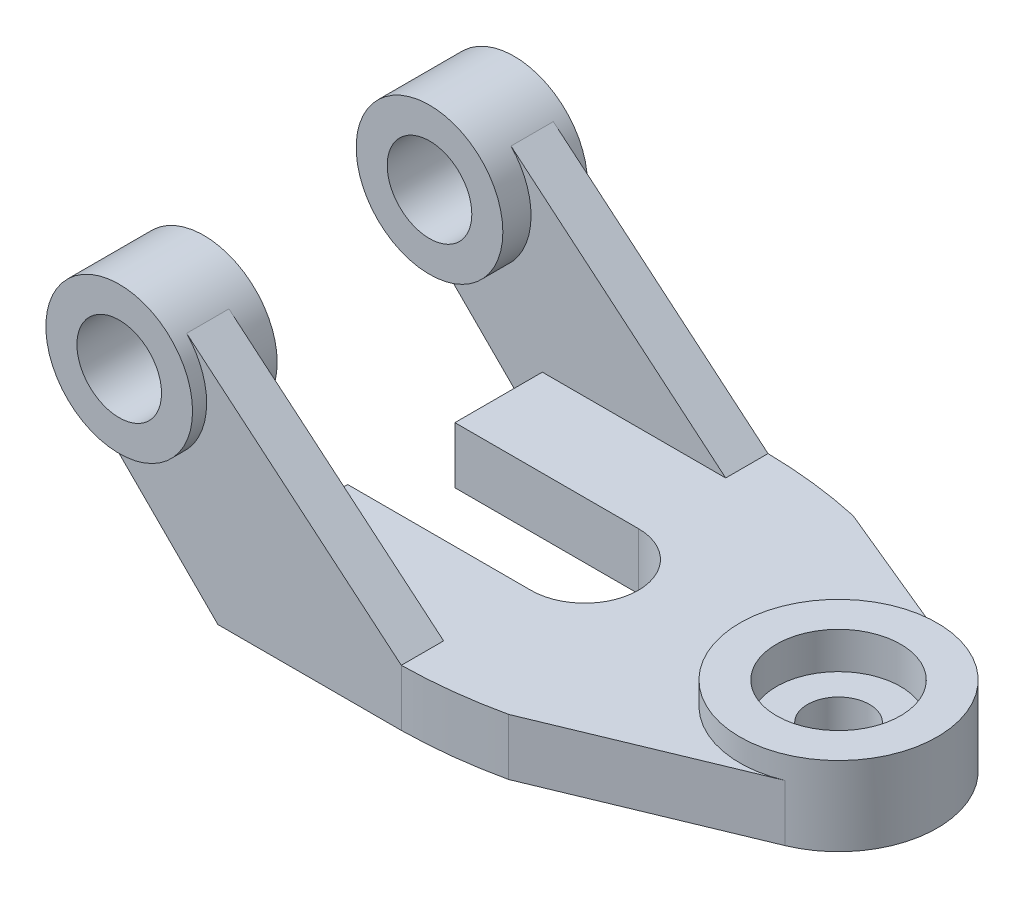
ISO-10303-21;
HEADER;
FILE_DESCRIPTION(('STEP AP214'),'2;1');
FILE_NAME('part.step','',(''),(''),'','','');
FILE_SCHEMA(('AUTOMOTIVE_DESIGN { 1 0 10303 214 1 1 1 1 }'));
ENDSEC;
DATA;
#1=APPLICATION_CONTEXT('core data for automotive mechanical design processes');
#2=APPLICATION_PROTOCOL_DEFINITION('international standard','automotive_design',2000,#1);
#3=PRODUCT_CONTEXT('',#1,'mechanical');
#4=PRODUCT('Part','Part','',(#3));
#5=PRODUCT_RELATED_PRODUCT_CATEGORY('part','',(#4));
#6=PRODUCT_DEFINITION_FORMATION('','',#4);
#7=PRODUCT_DEFINITION_CONTEXT('part definition',#1,'design');
#8=PRODUCT_DEFINITION('design','',#6,#7);
#9=PRODUCT_DEFINITION_SHAPE('','',#8);
#10=(LENGTH_UNIT() NAMED_UNIT(*) SI_UNIT(.MILLI.,.METRE.));
#11=(NAMED_UNIT(*) PLANE_ANGLE_UNIT() SI_UNIT($,.RADIAN.));
#12=(NAMED_UNIT(*) SI_UNIT($,.STERADIAN.) SOLID_ANGLE_UNIT());
#13=UNCERTAINTY_MEASURE_WITH_UNIT(LENGTH_MEASURE(1.E-05),#10,'distance_accuracy_value','');
#14=(GEOMETRIC_REPRESENTATION_CONTEXT(3) GLOBAL_UNCERTAINTY_ASSIGNED_CONTEXT((#13)) GLOBAL_UNIT_ASSIGNED_CONTEXT((#10,
#11,#12)) REPRESENTATION_CONTEXT('',''));
#15=CARTESIAN_POINT('',(0.,0.,0.));
#16=DIRECTION('',(0.,0.,1.));
#17=DIRECTION('',(1.,0.,0.));
#18=AXIS2_PLACEMENT_3D('',#15,#16,#17);
#19=CARTESIAN_POINT('',(-30.,66.,-31.));
#20=DIRECTION('',(0.,0.,-1.));
#21=DIRECTION('',(-1.,0.,0.));
#22=AXIS2_PLACEMENT_3D('',#19,#20,#21);
#23=PLANE('',#22);
#24=CARTESIAN_POINT('',(-30.,66.,-31.));
#25=DIRECTION('',(0.,0.,-1.));
#26=DIRECTION('',(-1.,0.,0.));
#27=AXIS2_PLACEMENT_3D('',#24,#25,#26);
#28=CIRCLE('',#27,26.);
#29=CARTESIAN_POINT('',(-44.2583426132256,44.2583426132257,-31.));
#30=VERTEX_POINT('',#29);
#31=CARTESIAN_POINT('',(-11.1036065621983,83.8585081976016,-31.));
#32=VERTEX_POINT('',#31);
#33=EDGE_CURVE('E379',#30,#32,#28,.F.);
#34=ORIENTED_EDGE('',*,*,#33,.F.);
#35=DIRECTION('',(-0.707106781186546,0.707106781186549,0.));
#36=VECTOR('',#35,1.);
#37=CARTESIAN_POINT('',(0.,0.,-31.));
#38=LINE('',#37,#36);
#39=CARTESIAN_POINT('',(0.,0.,-31.));
#40=VERTEX_POINT('',#39);
#41=EDGE_CURVE('E358',#40,#30,#38,.T.);
#42=ORIENTED_EDGE('',*,*,#41,.F.);
#43=DIRECTION('',(0.,1.,0.));
#44=VECTOR('',#43,1.);
#45=CARTESIAN_POINT('',(0.,20.,-31.));
#46=LINE('',#45,#44);
#47=CARTESIAN_POINT('',(0.,20.,-31.));
#48=VERTEX_POINT('',#47);
#49=EDGE_CURVE('E203',#40,#48,#46,.T.);
#50=ORIENTED_EDGE('',*,*,#49,.T.);
#51=DIRECTION('',(-1.,0.,0.));
#52=VECTOR('',#51,1.);
#53=CARTESIAN_POINT('',(65.,20.,-31.));
#54=LINE('',#53,#52);
#55=CARTESIAN_POINT('',(65.,20.,-31.));
#56=VERTEX_POINT('',#55);
#57=EDGE_CURVE('E56',#56,#48,#54,.T.);
#58=ORIENTED_EDGE('',*,*,#57,.F.);
#59=DIRECTION('',(0.766044443118977,-0.64278760968654,0.));
#60=VECTOR('',#59,1.);
#61=CARTESIAN_POINT('',(65.,20.,-31.));
#62=LINE('',#61,#60);
#63=EDGE_CURVE('E349',#32,#56,#62,.T.);
#64=ORIENTED_EDGE('',*,*,#63,.F.);
#65=EDGE_LOOP('',(#34,#42,#50,#58,#64));
#66=FACE_BOUND('',#65,.T.);
#67=ADVANCED_FACE('F39',(#66),#23,.F.);
#68=CARTESIAN_POINT('',(0.,20.,0.));
#69=DIRECTION('',(1.,0.,0.));
#70=DIRECTION('',(0.,0.,-1.));
#71=AXIS2_PLACEMENT_3D('',#68,#69,#70);
#72=PLANE('',#71);
#73=ORIENTED_EDGE('',*,*,#49,.F.);
#74=DIRECTION('',(0.,0.,1.));
#75=VECTOR('',#74,1.);
#76=CARTESIAN_POINT('',(0.,0.,0.));
#77=LINE('',#76,#75);
#78=CARTESIAN_POINT('',(0.,0.,0.));
#79=VERTEX_POINT('',#78);
#80=EDGE_CURVE('E256',#40,#79,#77,.T.);
#81=ORIENTED_EDGE('',*,*,#80,.T.);
#82=DIRECTION('',(0.,-1.,0.));
#83=VECTOR('',#82,1.);
#84=CARTESIAN_POINT('',(0.,20.,0.));
#85=LINE('',#84,#83);
#86=CARTESIAN_POINT('',(0.,20.,0.));
#87=VERTEX_POINT('',#86);
#88=EDGE_CURVE('E235',#87,#79,#85,.T.);
#89=ORIENTED_EDGE('',*,*,#88,.F.);
#90=DIRECTION('',(0.,0.,1.));
#91=VECTOR('',#90,1.);
#92=CARTESIAN_POINT('',(0.,20.,0.));
#93=LINE('',#92,#91);
#94=EDGE_CURVE('E234',#48,#87,#93,.T.);
#95=ORIENTED_EDGE('',*,*,#94,.F.);
#96=EDGE_LOOP('',(#73,#81,#89,#95));
#97=FACE_BOUND('',#96,.T.);
#98=ADVANCED_FACE('F375',(#97),#72,.F.);
#99=CARTESIAN_POINT('',(0.,20.,38.));
#100=DIRECTION('',(1.,0.,0.));
#101=DIRECTION('',(0.,0.,-1.));
#102=AXIS2_PLACEMENT_3D('',#99,#100,#101);
#103=PLANE('',#102);
#104=DIRECTION('',(0.,-1.,0.));
#105=VECTOR('',#104,1.);
#106=CARTESIAN_POINT('',(0.,20.,69.));
#107=LINE('',#106,#105);
#108=CARTESIAN_POINT('',(0.,20.,69.));
#109=VERTEX_POINT('',#108);
#110=CARTESIAN_POINT('',(0.,0.,69.));
#111=VERTEX_POINT('',#110);
#112=EDGE_CURVE('E189',#109,#111,#107,.T.);
#113=ORIENTED_EDGE('',*,*,#112,.F.);
#114=DIRECTION('',(0.,0.,1.));
#115=VECTOR('',#114,1.);
#116=CARTESIAN_POINT('',(0.,20.,38.));
#117=LINE('',#116,#115);
#118=CARTESIAN_POINT('',(0.,20.,38.));
#119=VERTEX_POINT('',#118);
#120=EDGE_CURVE('E219',#119,#109,#117,.T.);
#121=ORIENTED_EDGE('',*,*,#120,.F.);
#122=DIRECTION('',(0.,-1.,0.));
#123=VECTOR('',#122,1.);
#124=CARTESIAN_POINT('',(0.,20.,38.));
#125=LINE('',#124,#123);
#126=CARTESIAN_POINT('',(0.,0.,38.));
#127=VERTEX_POINT('',#126);
#128=EDGE_CURVE('E283',#119,#127,#125,.T.);
#129=ORIENTED_EDGE('',*,*,#128,.T.);
#130=DIRECTION('',(0.,0.,1.));
#131=VECTOR('',#130,1.);
#132=CARTESIAN_POINT('',(0.,0.,38.));
#133=LINE('',#132,#131);
#134=EDGE_CURVE('E243',#127,#111,#133,.T.);
#135=ORIENTED_EDGE('',*,*,#134,.T.);
#136=EDGE_LOOP('',(#113,#121,#129,#135));
#137=FACE_BOUND('',#136,.T.);
#138=ADVANCED_FACE('F307',(#137),#103,.F.);
#139=CARTESIAN_POINT('',(0.,20.,0.));
#140=DIRECTION('',(0.,0.,-1.));
#141=DIRECTION('',(-1.,0.,0.));
#142=AXIS2_PLACEMENT_3D('',#139,#140,#141);
#143=PLANE('',#142);
#144=DIRECTION('',(1.,0.,0.));
#145=VECTOR('',#144,1.);
#146=CARTESIAN_POINT('',(0.,0.,0.));
#147=LINE('',#146,#145);
#148=CARTESIAN_POINT('',(65.,0.,0.));
#149=VERTEX_POINT('',#148);
#150=EDGE_CURVE('E209',#79,#149,#147,.T.);
#151=ORIENTED_EDGE('',*,*,#150,.T.);
#152=DIRECTION('',(0.,-1.,0.));
#153=VECTOR('',#152,1.);
#154=CARTESIAN_POINT('',(65.,20.,0.));
#155=LINE('',#154,#153);
#156=CARTESIAN_POINT('',(65.,20.,0.));
#157=VERTEX_POINT('',#156);
#158=EDGE_CURVE('E43',#157,#149,#155,.T.);
#159=ORIENTED_EDGE('',*,*,#158,.F.);
#160=DIRECTION('',(1.,0.,0.));
#161=VECTOR('',#160,1.);
#162=CARTESIAN_POINT('',(0.,20.,0.));
#163=LINE('',#162,#161);
#164=EDGE_CURVE('E215',#87,#157,#163,.T.);
#165=ORIENTED_EDGE('',*,*,#164,.F.);
#166=ORIENTED_EDGE('',*,*,#88,.T.);
#167=EDGE_LOOP('',(#151,#159,#165,#166));
#168=FACE_BOUND('',#167,.T.);
#169=ADVANCED_FACE('F41',(#168),#143,.F.);
#170=CARTESIAN_POINT('',(65.,20.,19.));
#171=DIRECTION('',(0.,-1.,0.));
#172=DIRECTION('',(0.,0.,-1.));
#173=AXIS2_PLACEMENT_3D('',#170,#171,#172);
#174=CYLINDRICAL_SURFACE('',#173,19.);
#175=CARTESIAN_POINT('',(65.,0.,19.));
#176=DIRECTION('',(0.,-1.,0.));
#177=DIRECTION('',(0.,0.,1.));
#178=AXIS2_PLACEMENT_3D('',#175,#176,#177);
#179=CIRCLE('',#178,19.);
#180=CARTESIAN_POINT('',(65.,0.,38.));
#181=VERTEX_POINT('',#180);
#182=EDGE_CURVE('E240',#149,#181,#179,.T.);
#183=ORIENTED_EDGE('',*,*,#182,.T.);
#184=DIRECTION('',(0.,-1.,0.));
#185=VECTOR('',#184,1.);
#186=CARTESIAN_POINT('',(65.,20.,38.));
#187=LINE('',#186,#185);
#188=CARTESIAN_POINT('',(65.,20.,38.));
#189=VERTEX_POINT('',#188);
#190=EDGE_CURVE('E281',#189,#181,#187,.T.);
#191=ORIENTED_EDGE('',*,*,#190,.F.);
#192=CARTESIAN_POINT('',(65.,20.,19.));
#193=DIRECTION('',(0.,-1.,0.));
#194=DIRECTION('',(0.,0.,1.));
#195=AXIS2_PLACEMENT_3D('',#192,#193,#194);
#196=CIRCLE('',#195,19.);
#197=EDGE_CURVE('E214',#157,#189,#196,.T.);
#198=ORIENTED_EDGE('',*,*,#197,.F.);
#199=ORIENTED_EDGE('',*,*,#158,.T.);
#200=EDGE_LOOP('',(#183,#191,#198,#199));
#201=FACE_BOUND('',#200,.T.);
#202=ADVANCED_FACE('F295',(#201),#174,.F.);
#203=CARTESIAN_POINT('',(65.,20.,38.));
#204=DIRECTION('',(0.,0.,1.));
#205=DIRECTION('',(1.,0.,0.));
#206=AXIS2_PLACEMENT_3D('',#203,#204,#205);
#207=PLANE('',#206);
#208=DIRECTION('',(-1.,0.,0.));
#209=VECTOR('',#208,1.);
#210=CARTESIAN_POINT('',(65.,0.,38.));
#211=LINE('',#210,#209);
#212=EDGE_CURVE('E239',#181,#127,#211,.T.);
#213=ORIENTED_EDGE('',*,*,#212,.T.);
#214=ORIENTED_EDGE('',*,*,#128,.F.);
#215=DIRECTION('',(-1.,0.,0.));
#216=VECTOR('',#215,1.);
#217=CARTESIAN_POINT('',(65.,20.,38.));
#218=LINE('',#217,#216);
#219=EDGE_CURVE('E217',#189,#119,#218,.T.);
#220=ORIENTED_EDGE('',*,*,#219,.F.);
#221=ORIENTED_EDGE('',*,*,#190,.T.);
#222=EDGE_LOOP('',(#213,#214,#220,#221));
#223=FACE_BOUND('',#222,.T.);
#224=ADVANCED_FACE('F305',(#223),#207,.F.);
#225=CARTESIAN_POINT('',(0.,20.,84.));
#226=DIRECTION('',(0.,0.,-1.));
#227=DIRECTION('',(-1.,0.,0.));
#228=AXIS2_PLACEMENT_3D('',#225,#226,#227);
#229=PLANE('',#228);
#230=DIRECTION('',(-0.766044443118977,0.64278760968654,0.));
#231=VECTOR('',#230,1.);
#232=CARTESIAN_POINT('',(65.,20.,84.));
#233=LINE('',#232,#231);
#234=CARTESIAN_POINT('',(65.,20.,84.));
#235=VERTEX_POINT('',#234);
#236=CARTESIAN_POINT('',(-11.1036065621983,83.8585081976016,84.));
#237=VERTEX_POINT('',#236);
#238=EDGE_CURVE('E196',#235,#237,#233,.T.);
#239=ORIENTED_EDGE('',*,*,#238,.T.);
#240=CARTESIAN_POINT('',(-30.,66.,84.));
#241=DIRECTION('',(0.,0.,-1.));
#242=DIRECTION('',(-1.,0.,0.));
#243=AXIS2_PLACEMENT_3D('',#240,#241,#242);
#244=CIRCLE('',#243,26.);
#245=CARTESIAN_POINT('',(-44.2583426132256,44.2583426132258,84.));
#246=VERTEX_POINT('',#245);
#247=EDGE_CURVE('E174',#237,#246,#244,.T.);
#248=ORIENTED_EDGE('',*,*,#247,.T.);
#249=DIRECTION('',(0.707106781186546,-0.707106781186549,0.));
#250=VECTOR('',#249,1.);
#251=CARTESIAN_POINT('',(0.,0.,84.));
#252=LINE('',#251,#250);
#253=CARTESIAN_POINT('',(0.,0.,84.));
#254=VERTEX_POINT('',#253);
#255=EDGE_CURVE('E184',#246,#254,#252,.T.);
#256=ORIENTED_EDGE('',*,*,#255,.T.);
#257=DIRECTION('',(1.,0.,0.));
#258=VECTOR('',#257,1.);
#259=CARTESIAN_POINT('',(0.,0.,84.));
#260=LINE('',#259,#258);
#261=CARTESIAN_POINT('',(65.,0.,84.));
#262=VERTEX_POINT('',#261);
#263=EDGE_CURVE('E242',#254,#262,#260,.T.);
#264=ORIENTED_EDGE('',*,*,#263,.T.);
#265=DIRECTION('',(0.,-1.,0.));
#266=VECTOR('',#265,1.);
#267=CARTESIAN_POINT('',(65.,20.,84.));
#268=LINE('',#267,#266);
#269=EDGE_CURVE('E279',#235,#262,#268,.T.);
#270=ORIENTED_EDGE('',*,*,#269,.F.);
#271=EDGE_LOOP('',(#239,#248,#256,#264,#270));
#272=FACE_BOUND('',#271,.T.);
#273=ADVANCED_FACE('F320',(#272),#229,.F.);
#274=CARTESIAN_POINT('',(62.5288493474798,20.,-85.9820385054038));
#275=DIRECTION('',(0.,-1.,0.));
#276=DIRECTION('',(0.,0.,-1.));
#277=AXIS2_PLACEMENT_3D('',#274,#275,#276);
#278=CYLINDRICAL_SURFACE('',#277,170.);
#279=CARTESIAN_POINT('',(62.5288493474798,0.,-85.9820385054038));
#280=DIRECTION('',(0.,1.,0.));
#281=DIRECTION('',(0.,0.,1.));
#282=AXIS2_PLACEMENT_3D('',#279,#280,#281);
#283=CIRCLE('',#282,170.);
#284=CARTESIAN_POINT('',(99.1029551944317,0.,80.0370410652768));
#285=VERTEX_POINT('',#284);
#286=EDGE_CURVE('E248',#262,#285,#283,.T.);
#287=ORIENTED_EDGE('',*,*,#286,.T.);
#288=DIRECTION('',(0.,-1.,0.));
#289=VECTOR('',#288,1.);
#290=CARTESIAN_POINT('',(99.1029551944317,20.,80.0370410652768));
#291=LINE('',#290,#289);
#292=CARTESIAN_POINT('',(99.1029551944317,20.,80.0370410652768));
#293=VERTEX_POINT('',#292);
#294=EDGE_CURVE('E274',#293,#285,#291,.T.);
#295=ORIENTED_EDGE('',*,*,#294,.F.);
#296=CARTESIAN_POINT('',(62.5288493474798,20.,-85.9820385054038));
#297=DIRECTION('',(0.,1.,0.));
#298=DIRECTION('',(0.,0.,1.));
#299=AXIS2_PLACEMENT_3D('',#296,#297,#298);
#300=CIRCLE('',#299,170.);
#301=EDGE_CURVE('E224',#235,#293,#300,.T.);
#302=ORIENTED_EDGE('',*,*,#301,.F.);
#303=ORIENTED_EDGE('',*,*,#269,.T.);
#304=EDGE_LOOP('',(#287,#295,#302,#303));
#305=FACE_BOUND('',#304,.T.);
#306=ADVANCED_FACE('F319',(#305),#278,.T.);
#307=CARTESIAN_POINT('',(168.393920132778,20.,51.335783637895));
#308=DIRECTION('',(-0.382683432365091,0.,-0.923879532511287));
#309=DIRECTION('',(-0.923879532511287,0.,0.382683432365091));
#310=AXIS2_PLACEMENT_3D('',#307,#308,#309);
#311=PLANE('',#310);
#312=DIRECTION('',(0.923879532511286,0.,-0.382683432365091));
#313=VECTOR('',#312,1.);
#314=CARTESIAN_POINT('',(168.393920132778,0.,51.335783637895));
#315=LINE('',#314,#313);
#316=CARTESIAN_POINT('',(168.393920132778,0.,51.335783637895));
#317=VERTEX_POINT('',#316);
#318=EDGE_CURVE('E247',#285,#317,#315,.T.);
#319=ORIENTED_EDGE('',*,*,#318,.T.);
#320=DIRECTION('',(0.,-1.,0.));
#321=VECTOR('',#320,1.);
#322=CARTESIAN_POINT('',(168.393920132778,20.,51.335783637895));
#323=LINE('',#322,#321);
#324=CARTESIAN_POINT('',(168.393920132778,20.,51.335783637895));
#325=VERTEX_POINT('',#324);
#326=EDGE_CURVE('E275',#325,#317,#323,.T.);
#327=ORIENTED_EDGE('',*,*,#326,.F.);
#328=DIRECTION('',(0.923879532511286,0.,-0.382683432365091));
#329=VECTOR('',#328,1.);
#330=CARTESIAN_POINT('',(168.393920132778,20.,51.335783637895));
#331=LINE('',#330,#329);
#332=EDGE_CURVE('E223',#293,#325,#331,.T.);
#333=ORIENTED_EDGE('',*,*,#332,.F.);
#334=ORIENTED_EDGE('',*,*,#294,.T.);
#335=EDGE_LOOP('',(#319,#327,#333,#334));
#336=FACE_BOUND('',#335,.T.);
#337=ADVANCED_FACE('F322',(#336),#311,.F.);
#338=CARTESIAN_POINT('',(155.,20.,19.));
#339=DIRECTION('',(0.,-1.,0.));
#340=DIRECTION('',(0.,0.,-1.));
#341=AXIS2_PLACEMENT_3D('',#338,#339,#340);
#342=CYLINDRICAL_SURFACE('',#341,35.);
#343=CARTESIAN_POINT('',(155.,0.,19.));
#344=DIRECTION('',(0.,1.,0.));
#345=DIRECTION('',(0.,0.,1.));
#346=AXIS2_PLACEMENT_3D('',#343,#344,#345);
#347=CIRCLE('',#346,35.);
#348=CARTESIAN_POINT('',(168.393920132778,0.,-13.335783637895));
#349=VERTEX_POINT('',#348);
#350=EDGE_CURVE('E246',#317,#349,#347,.T.);
#351=ORIENTED_EDGE('',*,*,#350,.T.);
#352=DIRECTION('',(0.,-1.,0.));
#353=VECTOR('',#352,1.);
#354=CARTESIAN_POINT('',(168.393920132778,20.,-13.335783637895));
#355=LINE('',#354,#353);
#356=CARTESIAN_POINT('',(168.393920132778,20.,-13.335783637895));
#357=VERTEX_POINT('',#356);
#358=EDGE_CURVE('E267',#357,#349,#355,.T.);
#359=ORIENTED_EDGE('',*,*,#358,.F.);
#360=CARTESIAN_POINT('',(155.,20.,19.));
#361=DIRECTION('',(0.,1.,0.));
#362=DIRECTION('',(0.,0.,1.));
#363=AXIS2_PLACEMENT_3D('',#360,#361,#362);
#364=CIRCLE('',#363,35.);
#365=EDGE_CURVE('E11',#357,#325,#364,.T.);
#366=ORIENTED_EDGE('',*,*,#365,.T.);
#367=ORIENTED_EDGE('',*,*,#326,.T.);
#368=EDGE_LOOP('',(#351,#359,#366,#367));
#369=FACE_BOUND('',#368,.T.);
#370=CARTESIAN_POINT('',(155.,28.,19.));
#371=DIRECTION('',(0.,1.,0.));
#372=DIRECTION('',(0.,0.,1.));
#373=AXIS2_PLACEMENT_3D('',#370,#371,#372);
#374=CIRCLE('',#373,35.);
#375=CARTESIAN_POINT('',(155.,28.,54.));
#376=VERTEX_POINT('',#375);
#377=EDGE_CURVE('E208',#376,#376,#374,.T.);
#378=ORIENTED_EDGE('',*,*,#377,.F.);
#379=EDGE_LOOP('',(#378));
#380=FACE_BOUND('',#379,.T.);
#381=ADVANCED_FACE('F330',(#369,#380),#342,.T.);
#382=CARTESIAN_POINT('',(168.393920132778,20.,-13.335783637895));
#383=DIRECTION('',(-0.382683432365091,0.,0.923879532511286));
#384=DIRECTION('',(0.923879532511286,0.,0.382683432365091));
#385=AXIS2_PLACEMENT_3D('',#382,#383,#384);
#386=PLANE('',#385);
#387=DIRECTION('',(-0.923879532511286,0.,-0.382683432365091));
#388=VECTOR('',#387,1.);
#389=CARTESIAN_POINT('',(168.393920132778,0.,-13.335783637895));
#390=LINE('',#389,#388);
#391=CARTESIAN_POINT('',(99.1029551944317,0.,-42.0370410652768));
#392=VERTEX_POINT('',#391);
#393=EDGE_CURVE('E252',#349,#392,#390,.T.);
#394=ORIENTED_EDGE('',*,*,#393,.T.);
#395=DIRECTION('',(0.,-1.,0.));
#396=VECTOR('',#395,1.);
#397=CARTESIAN_POINT('',(99.1029551944317,20.,-42.0370410652768));
#398=LINE('',#397,#396);
#399=CARTESIAN_POINT('',(99.1029551944317,20.,-42.0370410652768));
#400=VERTEX_POINT('',#399);
#401=EDGE_CURVE('E266',#400,#392,#398,.T.);
#402=ORIENTED_EDGE('',*,*,#401,.F.);
#403=DIRECTION('',(-0.923879532511286,0.,-0.382683432365091));
#404=VECTOR('',#403,1.);
#405=CARTESIAN_POINT('',(168.393920132778,20.,-13.335783637895));
#406=LINE('',#405,#404);
#407=EDGE_CURVE('E226',#357,#400,#406,.T.);
#408=ORIENTED_EDGE('',*,*,#407,.F.);
#409=ORIENTED_EDGE('',*,*,#358,.T.);
#410=EDGE_LOOP('',(#394,#402,#408,#409));
#411=FACE_BOUND('',#410,.T.);
#412=ADVANCED_FACE('F331',(#411),#386,.F.);
#413=CARTESIAN_POINT('',(62.5288493474796,20.,123.982038505404));
#414=DIRECTION('',(0.,-1.,0.));
#415=DIRECTION('',(0.,0.,-1.));
#416=AXIS2_PLACEMENT_3D('',#413,#414,#415);
#417=CYLINDRICAL_SURFACE('',#416,170.);
#418=CARTESIAN_POINT('',(62.5288493474796,0.,123.982038505404));
#419=DIRECTION('',(0.,1.,0.));
#420=DIRECTION('',(0.,0.,-1.));
#421=AXIS2_PLACEMENT_3D('',#418,#419,#420);
#422=CIRCLE('',#421,170.);
#423=CARTESIAN_POINT('',(65.,0.,-46.));
#424=VERTEX_POINT('',#423);
#425=EDGE_CURVE('E255',#392,#424,#422,.T.);
#426=ORIENTED_EDGE('',*,*,#425,.T.);
#427=DIRECTION('',(0.,-1.,0.));
#428=VECTOR('',#427,1.);
#429=CARTESIAN_POINT('',(65.,20.,-46.));
#430=LINE('',#429,#428);
#431=CARTESIAN_POINT('',(65.,20.,-46.));
#432=VERTEX_POINT('',#431);
#433=EDGE_CURVE('E263',#432,#424,#430,.T.);
#434=ORIENTED_EDGE('',*,*,#433,.F.);
#435=CARTESIAN_POINT('',(62.5288493474796,20.,123.982038505404));
#436=DIRECTION('',(0.,1.,0.));
#437=DIRECTION('',(0.,0.,-1.));
#438=AXIS2_PLACEMENT_3D('',#435,#436,#437);
#439=CIRCLE('',#438,170.);
#440=EDGE_CURVE('E229',#400,#432,#439,.T.);
#441=ORIENTED_EDGE('',*,*,#440,.F.);
#442=ORIENTED_EDGE('',*,*,#401,.T.);
#443=EDGE_LOOP('',(#426,#434,#441,#442));
#444=FACE_BOUND('',#443,.T.);
#445=ADVANCED_FACE('F336',(#444),#417,.T.);
#446=CARTESIAN_POINT('',(0.,20.,-46.));
#447=DIRECTION('',(0.,0.,1.));
#448=DIRECTION('',(1.,0.,0.));
#449=AXIS2_PLACEMENT_3D('',#446,#447,#448);
#450=PLANE('',#449);
#451=CARTESIAN_POINT('',(-30.,66.,-46.));
#452=DIRECTION('',(0.,0.,1.));
#453=DIRECTION('',(1.,0.,0.));
#454=AXIS2_PLACEMENT_3D('',#451,#452,#453);
#455=CIRCLE('',#454,26.);
#456=CARTESIAN_POINT('',(-11.1036065621983,83.8585081976016,-46.));
#457=VERTEX_POINT('',#456);
#458=CARTESIAN_POINT('',(-44.2583426132256,44.2583426132257,-46.));
#459=VERTEX_POINT('',#458);
#460=EDGE_CURVE('E352',#457,#459,#455,.F.);
#461=ORIENTED_EDGE('',*,*,#460,.F.);
#462=DIRECTION('',(0.766044443118977,-0.64278760968654,0.));
#463=VECTOR('',#462,1.);
#464=CARTESIAN_POINT('',(65.,20.,-46.));
#465=LINE('',#464,#463);
#466=EDGE_CURVE('E350',#457,#432,#465,.T.);
#467=ORIENTED_EDGE('',*,*,#466,.T.);
#468=ORIENTED_EDGE('',*,*,#433,.T.);
#469=DIRECTION('',(-1.,0.,0.));
#470=VECTOR('',#469,1.);
#471=CARTESIAN_POINT('',(0.,0.,-46.));
#472=LINE('',#471,#470);
#473=CARTESIAN_POINT('',(0.,0.,-46.));
#474=VERTEX_POINT('',#473);
#475=EDGE_CURVE('E258',#424,#474,#472,.T.);
#476=ORIENTED_EDGE('',*,*,#475,.T.);
#477=DIRECTION('',(-0.707106781186546,0.707106781186549,0.));
#478=VECTOR('',#477,1.);
#479=CARTESIAN_POINT('',(0.,0.,-46.));
#480=LINE('',#479,#478);
#481=EDGE_CURVE('E359',#474,#459,#480,.T.);
#482=ORIENTED_EDGE('',*,*,#481,.T.);
#483=EDGE_LOOP('',(#461,#467,#468,#476,#482));
#484=FACE_BOUND('',#483,.T.);
#485=ADVANCED_FACE('F355',(#484),#450,.F.);
#486=CARTESIAN_POINT('',(65.,20.,19.));
#487=DIRECTION('',(0.,1.,0.));
#488=DIRECTION('',(0.,0.,1.));
#489=AXIS2_PLACEMENT_3D('',#486,#487,#488);
#490=PLANE('',#489);
#491=DIRECTION('',(0.,0.,-1.));
#492=VECTOR('',#491,1.);
#493=CARTESIAN_POINT('',(65.,20.,-31.));
#494=LINE('',#493,#492);
#495=EDGE_CURVE('E54',#56,#432,#494,.T.);
#496=ORIENTED_EDGE('',*,*,#495,.F.);
#497=ORIENTED_EDGE('',*,*,#57,.T.);
#498=ORIENTED_EDGE('',*,*,#94,.T.);
#499=ORIENTED_EDGE('',*,*,#164,.T.);
#500=ORIENTED_EDGE('',*,*,#197,.T.);
#501=ORIENTED_EDGE('',*,*,#219,.T.);
#502=ORIENTED_EDGE('',*,*,#120,.T.);
#503=DIRECTION('',(1.,0.,0.));
#504=VECTOR('',#503,1.);
#505=CARTESIAN_POINT('',(65.,20.,69.));
#506=LINE('',#505,#504);
#507=CARTESIAN_POINT('',(65.,20.,69.));
#508=VERTEX_POINT('',#507);
#509=EDGE_CURVE('E201',#109,#508,#506,.T.);
#510=ORIENTED_EDGE('',*,*,#509,.T.);
#511=DIRECTION('',(0.,0.,1.));
#512=VECTOR('',#511,1.);
#513=CARTESIAN_POINT('',(65.,20.,69.));
#514=LINE('',#513,#512);
#515=EDGE_CURVE('E193',#508,#235,#514,.T.);
#516=ORIENTED_EDGE('',*,*,#515,.T.);
#517=ORIENTED_EDGE('',*,*,#301,.T.);
#518=ORIENTED_EDGE('',*,*,#332,.T.);
#519=ORIENTED_EDGE('',*,*,#365,.F.);
#520=ORIENTED_EDGE('',*,*,#407,.T.);
#521=ORIENTED_EDGE('',*,*,#440,.T.);
#522=EDGE_LOOP('',(#496,#497,#498,#499,#500,#501,#502,#510,#516,#517,#518,#519,#520,#521));
#523=FACE_BOUND('',#522,.T.);
#524=ADVANCED_FACE('F306',(#523),#490,.T.);
#525=CARTESIAN_POINT('',(65.,0.,19.));
#526=DIRECTION('',(0.,1.,0.));
#527=DIRECTION('',(0.,0.,1.));
#528=AXIS2_PLACEMENT_3D('',#525,#526,#527);
#529=PLANE('',#528);
#530=CARTESIAN_POINT('',(155.,0.,19.));
#531=DIRECTION('',(0.,1.,0.));
#532=DIRECTION('',(0.,0.,1.));
#533=AXIS2_PLACEMENT_3D('',#530,#531,#532);
#534=CIRCLE('',#533,11.);
#535=CARTESIAN_POINT('',(155.,0.,30.));
#536=VERTEX_POINT('',#535);
#537=EDGE_CURVE('E414',#536,#536,#534,.T.);
#538=ORIENTED_EDGE('',*,*,#537,.T.);
#539=EDGE_LOOP('',(#538));
#540=FACE_BOUND('',#539,.T.);
#541=ORIENTED_EDGE('',*,*,#475,.F.);
#542=ORIENTED_EDGE('',*,*,#425,.F.);
#543=ORIENTED_EDGE('',*,*,#393,.F.);
#544=ORIENTED_EDGE('',*,*,#350,.F.);
#545=ORIENTED_EDGE('',*,*,#318,.F.);
#546=ORIENTED_EDGE('',*,*,#286,.F.);
#547=ORIENTED_EDGE('',*,*,#263,.F.);
#548=DIRECTION('',(0.,0.,1.));
#549=VECTOR('',#548,1.);
#550=CARTESIAN_POINT('',(0.,0.,69.));
#551=LINE('',#550,#549);
#552=EDGE_CURVE('E183',#111,#254,#551,.T.);
#553=ORIENTED_EDGE('',*,*,#552,.F.);
#554=ORIENTED_EDGE('',*,*,#134,.F.);
#555=ORIENTED_EDGE('',*,*,#212,.F.);
#556=ORIENTED_EDGE('',*,*,#182,.F.);
#557=ORIENTED_EDGE('',*,*,#150,.F.);
#558=ORIENTED_EDGE('',*,*,#80,.F.);
#559=EDGE_CURVE('E216',#474,#40,#77,.T.);
#560=ORIENTED_EDGE('',*,*,#559,.F.);
#561=EDGE_LOOP('',(#541,#542,#543,#544,#545,#546,#547,#553,#554,#555,#556,#557,#558,#560));
#562=FACE_BOUND('',#561,.T.);
#563=ADVANCED_FACE('F297',(#540,#562),#529,.F.);
#564=CARTESIAN_POINT('',(155.,28.,19.));
#565=DIRECTION('',(0.,1.,0.));
#566=DIRECTION('',(0.,0.,1.));
#567=AXIS2_PLACEMENT_3D('',#564,#565,#566);
#568=PLANE('',#567);
#569=CARTESIAN_POINT('',(155.,28.,19.));
#570=DIRECTION('',(0.,1.,0.));
#571=DIRECTION('',(0.,0.,1.));
#572=AXIS2_PLACEMENT_3D('',#569,#570,#571);
#573=CIRCLE('',#572,22.);
#574=CARTESIAN_POINT('',(155.,28.,41.));
#575=VERTEX_POINT('',#574);
#576=EDGE_CURVE('E407',#575,#575,#573,.T.);
#577=ORIENTED_EDGE('',*,*,#576,.F.);
#578=EDGE_LOOP('',(#577));
#579=FACE_BOUND('',#578,.T.);
#580=ORIENTED_EDGE('',*,*,#377,.T.);
#581=EDGE_LOOP('',(#580));
#582=FACE_BOUND('',#581,.T.);
#583=ADVANCED_FACE('F442',(#579,#582),#568,.T.);
#584=CARTESIAN_POINT('',(-30.,66.,69.));
#585=DIRECTION('',(0.,0.,1.));
#586=DIRECTION('',(1.,0.,0.));
#587=AXIS2_PLACEMENT_3D('',#584,#585,#586);
#588=PLANE('',#587);
#589=DIRECTION('',(0.707106781186546,-0.707106781186549,0.));
#590=VECTOR('',#589,1.);
#591=CARTESIAN_POINT('',(0.,0.,69.));
#592=LINE('',#591,#590);
#593=CARTESIAN_POINT('',(-44.2583426132256,44.2583426132258,69.));
#594=VERTEX_POINT('',#593);
#595=EDGE_CURVE('E185',#594,#111,#592,.T.);
#596=ORIENTED_EDGE('',*,*,#595,.F.);
#597=CARTESIAN_POINT('',(-30.,66.,69.));
#598=DIRECTION('',(0.,0.,1.));
#599=DIRECTION('',(1.,0.,0.));
#600=AXIS2_PLACEMENT_3D('',#597,#598,#599);
#601=CIRCLE('',#600,26.);
#602=CARTESIAN_POINT('',(-11.1036065621983,83.8585081976016,69.));
#603=VERTEX_POINT('',#602);
#604=EDGE_CURVE('E162',#594,#603,#601,.T.);
#605=ORIENTED_EDGE('',*,*,#604,.T.);
#606=DIRECTION('',(-0.766044443118977,0.64278760968654,0.));
#607=VECTOR('',#606,1.);
#608=CARTESIAN_POINT('',(65.,20.,69.));
#609=LINE('',#608,#607);
#610=EDGE_CURVE('E194',#508,#603,#609,.T.);
#611=ORIENTED_EDGE('',*,*,#610,.F.);
#612=ORIENTED_EDGE('',*,*,#509,.F.);
#613=ORIENTED_EDGE('',*,*,#112,.T.);
#614=EDGE_LOOP('',(#596,#605,#611,#612,#613));
#615=FACE_BOUND('',#614,.T.);
#616=ADVANCED_FACE('F186',(#615),#588,.F.);
#617=CARTESIAN_POINT('',(0.,0.,69.));
#618=DIRECTION('',(-0.707106781186549,-0.707106781186546,0.));
#619=DIRECTION('',(0.707106781186546,-0.707106781186549,0.));
#620=AXIS2_PLACEMENT_3D('',#617,#618,#619);
#621=PLANE('',#620);
#622=ORIENTED_EDGE('',*,*,#255,.F.);
#623=DIRECTION('',(0.,0.,1.));
#624=VECTOR('',#623,1.);
#625=CARTESIAN_POINT('',(-44.2583426132256,44.2583426132258,69.));
#626=LINE('',#625,#624);
#627=EDGE_CURVE('E169',#594,#246,#626,.T.);
#628=ORIENTED_EDGE('',*,*,#627,.F.);
#629=ORIENTED_EDGE('',*,*,#595,.T.);
#630=ORIENTED_EDGE('',*,*,#552,.T.);
#631=EDGE_LOOP('',(#622,#628,#629,#630));
#632=FACE_BOUND('',#631,.T.);
#633=ADVANCED_FACE('F176',(#632),#621,.T.);
#634=CARTESIAN_POINT('',(-30.,66.,69.));
#635=DIRECTION('',(0.,0.,1.));
#636=DIRECTION('',(1.,0.,0.));
#637=AXIS2_PLACEMENT_3D('',#634,#635,#636);
#638=CYLINDRICAL_SURFACE('',#637,26.);
#639=ORIENTED_EDGE('',*,*,#627,.T.);
#640=ORIENTED_EDGE('',*,*,#247,.F.);
#641=DIRECTION('',(0.,0.,1.));
#642=VECTOR('',#641,1.);
#643=CARTESIAN_POINT('',(-11.1036065621983,83.8585081976016,69.));
#644=LINE('',#643,#642);
#645=EDGE_CURVE('E168',#603,#237,#644,.T.);
#646=ORIENTED_EDGE('',*,*,#645,.F.);
#647=ORIENTED_EDGE('',*,*,#604,.F.);
#648=EDGE_LOOP('',(#639,#640,#646,#647));
#649=FACE_BOUND('',#648,.T.);
#650=CARTESIAN_POINT('',(-30.,66.,59.));
#651=DIRECTION('',(0.,0.,1.));
#652=DIRECTION('',(1.,0.,0.));
#653=AXIS2_PLACEMENT_3D('',#650,#651,#652);
#654=CIRCLE('',#653,26.);
#655=CARTESIAN_POINT('',(-4.00000000000001,66.,59.));
#656=VERTEX_POINT('',#655);
#657=EDGE_CURVE('E178',#656,#656,#654,.T.);
#658=ORIENTED_EDGE('',*,*,#657,.T.);
#659=EDGE_LOOP('',(#658));
#660=FACE_BOUND('',#659,.T.);
#661=CARTESIAN_POINT('',(-30.,66.,89.));
#662=DIRECTION('',(0.,0.,1.));
#663=DIRECTION('',(1.,0.,0.));
#664=AXIS2_PLACEMENT_3D('',#661,#662,#663);
#665=CIRCLE('',#664,26.);
#666=CARTESIAN_POINT('',(-4.00000000000001,66.,89.));
#667=VERTEX_POINT('',#666);
#668=EDGE_CURVE('E393',#667,#667,#665,.T.);
#669=ORIENTED_EDGE('',*,*,#668,.F.);
#670=EDGE_LOOP('',(#669));
#671=FACE_BOUND('',#670,.T.);
#672=ADVANCED_FACE('F164',(#649,#660,#671),#638,.T.);
#673=CARTESIAN_POINT('',(65.,20.,69.));
#674=DIRECTION('',(0.64278760968654,0.766044443118977,0.));
#675=DIRECTION('',(-0.766044443118977,0.64278760968654,0.));
#676=AXIS2_PLACEMENT_3D('',#673,#674,#675);
#677=PLANE('',#676);
#678=ORIENTED_EDGE('',*,*,#238,.F.);
#679=ORIENTED_EDGE('',*,*,#515,.F.);
#680=ORIENTED_EDGE('',*,*,#610,.T.);
#681=ORIENTED_EDGE('',*,*,#645,.T.);
#682=EDGE_LOOP('',(#678,#679,#680,#681));
#683=FACE_BOUND('',#682,.T.);
#684=ADVANCED_FACE('F315',(#683),#677,.T.);
#685=CARTESIAN_POINT('',(65.,20.,-31.));
#686=DIRECTION('',(0.64278760968654,0.766044443118977,0.));
#687=DIRECTION('',(-0.766044443118977,0.64278760968654,0.));
#688=AXIS2_PLACEMENT_3D('',#685,#686,#687);
#689=PLANE('',#688);
#690=ORIENTED_EDGE('',*,*,#466,.F.);
#691=DIRECTION('',(0.,0.,-1.));
#692=VECTOR('',#691,1.);
#693=CARTESIAN_POINT('',(-11.1036065621983,83.8585081976016,-31.));
#694=LINE('',#693,#692);
#695=EDGE_CURVE('E348',#32,#457,#694,.T.);
#696=ORIENTED_EDGE('',*,*,#695,.F.);
#697=ORIENTED_EDGE('',*,*,#63,.T.);
#698=ORIENTED_EDGE('',*,*,#495,.T.);
#699=EDGE_LOOP('',(#690,#696,#697,#698));
#700=FACE_BOUND('',#699,.T.);
#701=ADVANCED_FACE('F341',(#700),#689,.T.);
#702=CARTESIAN_POINT('',(-30.,66.,-31.));
#703=DIRECTION('',(0.,0.,-1.));
#704=DIRECTION('',(-1.,0.,0.));
#705=AXIS2_PLACEMENT_3D('',#702,#703,#704);
#706=CYLINDRICAL_SURFACE('',#705,26.);
#707=ORIENTED_EDGE('',*,*,#695,.T.);
#708=ORIENTED_EDGE('',*,*,#460,.T.);
#709=DIRECTION('',(0.,0.,-1.));
#710=VECTOR('',#709,1.);
#711=CARTESIAN_POINT('',(-44.2583426132256,44.2583426132258,-31.));
#712=LINE('',#711,#710);
#713=EDGE_CURVE('E364',#30,#459,#712,.T.);
#714=ORIENTED_EDGE('',*,*,#713,.F.);
#715=ORIENTED_EDGE('',*,*,#33,.T.);
#716=EDGE_LOOP('',(#707,#708,#714,#715));
#717=FACE_BOUND('',#716,.T.);
#718=CARTESIAN_POINT('',(-30.,66.,-21.));
#719=DIRECTION('',(0.,0.,1.));
#720=DIRECTION('',(1.,0.,0.));
#721=AXIS2_PLACEMENT_3D('',#718,#719,#720);
#722=CIRCLE('',#721,26.);
#723=CARTESIAN_POINT('',(-4.,66.,-21.));
#724=VERTEX_POINT('',#723);
#725=EDGE_CURVE('E385',#724,#724,#722,.T.);
#726=ORIENTED_EDGE('',*,*,#725,.F.);
#727=EDGE_LOOP('',(#726));
#728=FACE_BOUND('',#727,.T.);
#729=CARTESIAN_POINT('',(-30.,66.,-51.));
#730=DIRECTION('',(0.,0.,1.));
#731=DIRECTION('',(1.,0.,0.));
#732=AXIS2_PLACEMENT_3D('',#729,#730,#731);
#733=CIRCLE('',#732,26.);
#734=CARTESIAN_POINT('',(-4.,66.,-51.));
#735=VERTEX_POINT('',#734);
#736=EDGE_CURVE('E384',#735,#735,#733,.T.);
#737=ORIENTED_EDGE('',*,*,#736,.T.);
#738=EDGE_LOOP('',(#737));
#739=FACE_BOUND('',#738,.T.);
#740=ADVANCED_FACE('F378',(#717,#728,#739),#706,.T.);
#741=CARTESIAN_POINT('',(0.,0.,-31.));
#742=DIRECTION('',(-0.707106781186549,-0.707106781186546,0.));
#743=DIRECTION('',(0.707106781186546,-0.707106781186549,0.));
#744=AXIS2_PLACEMENT_3D('',#741,#742,#743);
#745=PLANE('',#744);
#746=ORIENTED_EDGE('',*,*,#481,.F.);
#747=ORIENTED_EDGE('',*,*,#559,.T.);
#748=ORIENTED_EDGE('',*,*,#41,.T.);
#749=ORIENTED_EDGE('',*,*,#713,.T.);
#750=EDGE_LOOP('',(#746,#747,#748,#749));
#751=FACE_BOUND('',#750,.T.);
#752=ADVANCED_FACE('F374',(#751),#745,.T.);
#753=CARTESIAN_POINT('',(-30.,66.,-21.));
#754=DIRECTION('',(0.,0.,1.));
#755=DIRECTION('',(1.,0.,0.));
#756=AXIS2_PLACEMENT_3D('',#753,#754,#755);
#757=PLANE('',#756);
#758=CARTESIAN_POINT('',(-30.,66.,-21.));
#759=DIRECTION('',(0.,0.,1.));
#760=DIRECTION('',(1.,0.,0.));
#761=AXIS2_PLACEMENT_3D('',#758,#759,#760);
#762=CIRCLE('',#761,15.);
#763=CARTESIAN_POINT('',(-15.,66.,-21.));
#764=VERTEX_POINT('',#763);
#765=EDGE_CURVE('E392',#764,#764,#762,.T.);
#766=ORIENTED_EDGE('',*,*,#765,.F.);
#767=EDGE_LOOP('',(#766));
#768=FACE_BOUND('',#767,.T.);
#769=ORIENTED_EDGE('',*,*,#725,.T.);
#770=EDGE_LOOP('',(#769));
#771=FACE_BOUND('',#770,.T.);
#772=ADVANCED_FACE('F472',(#768,#771),#757,.T.);
#773=CARTESIAN_POINT('',(-30.,66.,-51.));
#774=DIRECTION('',(0.,0.,1.));
#775=DIRECTION('',(1.,0.,0.));
#776=AXIS2_PLACEMENT_3D('',#773,#774,#775);
#777=PLANE('',#776);
#778=CARTESIAN_POINT('',(-30.,66.,-51.));
#779=DIRECTION('',(0.,0.,1.));
#780=DIRECTION('',(1.,0.,0.));
#781=AXIS2_PLACEMENT_3D('',#778,#779,#780);
#782=CIRCLE('',#781,15.);
#783=CARTESIAN_POINT('',(-15.,66.,-51.));
#784=VERTEX_POINT('',#783);
#785=EDGE_CURVE('E405',#784,#784,#782,.T.);
#786=ORIENTED_EDGE('',*,*,#785,.T.);
#787=EDGE_LOOP('',(#786));
#788=FACE_BOUND('',#787,.T.);
#789=ORIENTED_EDGE('',*,*,#736,.F.);
#790=EDGE_LOOP('',(#789));
#791=FACE_BOUND('',#790,.T.);
#792=ADVANCED_FACE('F462',(#788,#791),#777,.F.);
#793=CARTESIAN_POINT('',(-30.,66.,59.));
#794=DIRECTION('',(0.,0.,1.));
#795=DIRECTION('',(1.,0.,0.));
#796=AXIS2_PLACEMENT_3D('',#793,#794,#795);
#797=PLANE('',#796);
#798=CARTESIAN_POINT('',(-30.,66.,59.));
#799=DIRECTION('',(0.,0.,1.));
#800=DIRECTION('',(1.,0.,0.));
#801=AXIS2_PLACEMENT_3D('',#798,#799,#800);
#802=CIRCLE('',#801,15.);
#803=CARTESIAN_POINT('',(-15.,66.,59.));
#804=VERTEX_POINT('',#803);
#805=EDGE_CURVE('E400',#804,#804,#802,.T.);
#806=ORIENTED_EDGE('',*,*,#805,.T.);
#807=EDGE_LOOP('',(#806));
#808=FACE_BOUND('',#807,.T.);
#809=ORIENTED_EDGE('',*,*,#657,.F.);
#810=EDGE_LOOP('',(#809));
#811=FACE_BOUND('',#810,.T.);
#812=ADVANCED_FACE('F614',(#808,#811),#797,.F.);
#813=CARTESIAN_POINT('',(-30.,66.,89.));
#814=DIRECTION('',(0.,0.,1.));
#815=DIRECTION('',(1.,0.,0.));
#816=AXIS2_PLACEMENT_3D('',#813,#814,#815);
#817=PLANE('',#816);
#818=CARTESIAN_POINT('',(-30.,66.,89.));
#819=DIRECTION('',(0.,0.,1.));
#820=DIRECTION('',(1.,0.,0.));
#821=AXIS2_PLACEMENT_3D('',#818,#819,#820);
#822=CIRCLE('',#821,15.);
#823=CARTESIAN_POINT('',(-15.,66.,89.));
#824=VERTEX_POINT('',#823);
#825=EDGE_CURVE('E401',#824,#824,#822,.T.);
#826=ORIENTED_EDGE('',*,*,#825,.F.);
#827=EDGE_LOOP('',(#826));
#828=FACE_BOUND('',#827,.T.);
#829=ORIENTED_EDGE('',*,*,#668,.T.);
#830=EDGE_LOOP('',(#829));
#831=FACE_BOUND('',#830,.T.);
#832=ADVANCED_FACE('F625',(#828,#831),#817,.T.);
#833=CARTESIAN_POINT('',(-30.,66.,-51.));
#834=DIRECTION('',(0.,0.,1.));
#835=DIRECTION('',(1.,0.,0.));
#836=AXIS2_PLACEMENT_3D('',#833,#834,#835);
#837=CYLINDRICAL_SURFACE('',#836,15.);
#838=ORIENTED_EDGE('',*,*,#825,.T.);
#839=EDGE_LOOP('',(#838));
#840=FACE_BOUND('',#839,.T.);
#841=ORIENTED_EDGE('',*,*,#805,.F.);
#842=EDGE_LOOP('',(#841));
#843=FACE_BOUND('',#842,.T.);
#844=ADVANCED_FACE('F633',(#840,#843),#837,.F.);
#845=ORIENTED_EDGE('',*,*,#765,.T.);
#846=EDGE_LOOP('',(#845));
#847=FACE_BOUND('',#846,.T.);
#848=ORIENTED_EDGE('',*,*,#785,.F.);
#849=EDGE_LOOP('',(#848));
#850=FACE_BOUND('',#849,.T.);
#851=ADVANCED_FACE('F440',(#847,#850),#837,.F.);
#852=CARTESIAN_POINT('',(155.,15.,19.));
#853=DIRECTION('',(0.,1.,0.));
#854=DIRECTION('',(0.,0.,1.));
#855=AXIS2_PLACEMENT_3D('',#852,#853,#854);
#856=CYLINDRICAL_SURFACE('',#855,22.);
#857=CARTESIAN_POINT('',(155.,15.,19.));
#858=DIRECTION('',(0.,1.,0.));
#859=DIRECTION('',(0.,0.,1.));
#860=AXIS2_PLACEMENT_3D('',#857,#858,#859);
#861=CIRCLE('',#860,22.);
#862=CARTESIAN_POINT('',(155.,15.,41.));
#863=VERTEX_POINT('',#862);
#864=EDGE_CURVE('E408',#863,#863,#861,.T.);
#865=CARTESIAN_POINT('',(155.,15.,41.));
#866=CARTESIAN_POINT('',(155.,15.1354166666667,41.));
#867=CARTESIAN_POINT('',(155.,15.2708333333333,41.));
#868=CARTESIAN_POINT('',(155.,15.5416666666667,41.));
#869=CARTESIAN_POINT('',(155.,15.6770833333333,41.));
#870=CARTESIAN_POINT('',(155.,15.9479166666667,41.));
#871=CARTESIAN_POINT('',(155.,16.0833333333333,41.));
#872=CARTESIAN_POINT('',(155.,16.3541666666667,41.));
#873=CARTESIAN_POINT('',(155.,16.4895833333333,41.));
#874=CARTESIAN_POINT('',(155.,16.7604166666667,41.));
#875=CARTESIAN_POINT('',(155.,16.8958333333333,41.));
#876=CARTESIAN_POINT('',(155.,17.1666666666667,41.));
#877=CARTESIAN_POINT('',(155.,17.3020833333333,41.));
#878=CARTESIAN_POINT('',(155.,17.5729166666667,41.));
#879=CARTESIAN_POINT('',(155.,17.7083333333333,41.));
#880=CARTESIAN_POINT('',(155.,17.9791666666667,41.));
#881=CARTESIAN_POINT('',(155.,18.1145833333333,41.));
#882=CARTESIAN_POINT('',(155.,18.3854166666667,41.));
#883=CARTESIAN_POINT('',(155.,18.5208333333333,41.));
#884=CARTESIAN_POINT('',(155.,18.7916666666667,41.));
#885=CARTESIAN_POINT('',(155.,18.9270833333333,41.));
#886=CARTESIAN_POINT('',(155.,19.1979166666667,41.));
#887=CARTESIAN_POINT('',(155.,19.3333333333333,41.));
#888=CARTESIAN_POINT('',(155.,19.6041666666667,41.));
#889=CARTESIAN_POINT('',(155.,19.7395833333333,41.));
#890=CARTESIAN_POINT('',(155.,20.0104166666667,41.));
#891=CARTESIAN_POINT('',(155.,20.1458333333333,41.));
#892=CARTESIAN_POINT('',(155.,20.4166666666667,41.));
#893=CARTESIAN_POINT('',(155.,20.5520833333333,41.));
#894=CARTESIAN_POINT('',(155.,20.8229166666667,41.));
#895=CARTESIAN_POINT('',(155.,20.9583333333333,41.));
#896=CARTESIAN_POINT('',(155.,21.2291666666667,41.));
#897=CARTESIAN_POINT('',(155.,21.3645833333333,41.));
#898=CARTESIAN_POINT('',(155.,21.6354166666667,41.));
#899=CARTESIAN_POINT('',(155.,21.7708333333333,41.));
#900=CARTESIAN_POINT('',(155.,22.0416666666667,41.));
#901=CARTESIAN_POINT('',(155.,22.1770833333333,41.));
#902=CARTESIAN_POINT('',(155.,22.4479166666667,41.));
#903=CARTESIAN_POINT('',(155.,22.5833333333333,41.));
#904=CARTESIAN_POINT('',(155.,22.8541666666667,41.));
#905=CARTESIAN_POINT('',(155.,22.9895833333333,41.));
#906=CARTESIAN_POINT('',(155.,23.2604166666667,41.));
#907=CARTESIAN_POINT('',(155.,23.3958333333333,41.));
#908=CARTESIAN_POINT('',(155.,23.6666666666667,41.));
#909=CARTESIAN_POINT('',(155.,23.8020833333333,41.));
#910=CARTESIAN_POINT('',(155.,24.0729166666667,41.));
#911=CARTESIAN_POINT('',(155.,24.2083333333333,41.));
#912=CARTESIAN_POINT('',(155.,24.4791666666667,41.));
#913=CARTESIAN_POINT('',(155.,24.6145833333333,41.));
#914=CARTESIAN_POINT('',(155.,24.8854166666667,41.));
#915=CARTESIAN_POINT('',(155.,25.0208333333333,41.));
#916=CARTESIAN_POINT('',(155.,25.2916666666667,41.));
#917=CARTESIAN_POINT('',(155.,25.4270833333333,41.));
#918=CARTESIAN_POINT('',(155.,25.6979166666667,41.));
#919=CARTESIAN_POINT('',(155.,25.8333333333333,41.));
#920=CARTESIAN_POINT('',(155.,26.1041666666667,41.));
#921=CARTESIAN_POINT('',(155.,26.2395833333333,41.));
#922=CARTESIAN_POINT('',(155.,26.5104166666667,41.));
#923=CARTESIAN_POINT('',(155.,26.6458333333333,41.));
#924=CARTESIAN_POINT('',(155.,26.9166666666667,41.));
#925=CARTESIAN_POINT('',(155.,27.0520833333333,41.));
#926=CARTESIAN_POINT('',(155.,27.3229166666667,41.));
#927=CARTESIAN_POINT('',(155.,27.4583333333333,41.));
#928=CARTESIAN_POINT('',(155.,27.7291666666667,41.));
#929=CARTESIAN_POINT('',(155.,27.8645833333333,41.));
#930=CARTESIAN_POINT('',(155.,28.,41.));
#931=B_SPLINE_CURVE_WITH_KNOTS('',3,(#865,#866,#867,#868,#869,#870,#871,#872,#873,#874,#875,
#876,#877,#878,#879,#880,#881,#882,#883,#884,#885,#886,#887,#888,#889,#890,#891,#892,#893,#894,
#895,#896,#897,#898,#899,#900,#901,#902,#903,#904,#905,#906,#907,#908,#909,#910,#911,#912,#913,
#914,#915,#916,#917,#918,#919,#920,#921,#922,#923,#924,#925,#926,#927,#928,#929,#930),
.UNSPECIFIED.,.F.,.F.,(4,2,2,2,2,2,2,2,2,2,2,2,2,2,2,2,2,2,2,2,2,2,2,2,2,2,2,2,2,2,2,2,4),(0.,
0.40625,0.812500000000001,1.21875,1.625,2.03125,2.4375,2.84375,3.25,3.65625,4.0625,4.46875,
4.875,5.28125,5.6875,6.09375,6.5,6.90625,7.3125,7.71875,8.125,8.53125,8.9375,9.34375,9.75,
10.15625,10.5625,10.96875,11.375,11.78125,12.1875,12.59375,13.),.UNSPECIFIED.);
#932=EDGE_CURVE('BSEAM431',#863,#575,#931,.T.);
#933=ORIENTED_EDGE('',*,*,#864,.F.);
#934=ORIENTED_EDGE('',*,*,#576,.T.);
#935=ORIENTED_EDGE('',*,*,#932,.T.);
#936=ORIENTED_EDGE('',*,*,#932,.F.);
#937=EDGE_LOOP('',(#933,#935,#934,#936));
#938=FACE_BOUND('',#937,.T.);
#939=ADVANCED_FACE('F431',(#938),#856,.F.);
#940=CARTESIAN_POINT('',(155.,15.,19.));
#941=DIRECTION('',(0.,1.,0.));
#942=DIRECTION('',(0.,0.,1.));
#943=AXIS2_PLACEMENT_3D('',#940,#941,#942);
#944=PLANE('',#943);
#945=CARTESIAN_POINT('',(155.,15.,19.));
#946=DIRECTION('',(0.,1.,0.));
#947=DIRECTION('',(0.,0.,1.));
#948=AXIS2_PLACEMENT_3D('',#945,#946,#947);
#949=CIRCLE('',#948,11.);
#950=CARTESIAN_POINT('',(155.,15.,30.));
#951=VERTEX_POINT('',#950);
#952=EDGE_CURVE('E411',#951,#951,#949,.T.);
#953=ORIENTED_EDGE('',*,*,#952,.F.);
#954=EDGE_LOOP('',(#953));
#955=FACE_BOUND('',#954,.T.);
#956=ORIENTED_EDGE('',*,*,#864,.T.);
#957=EDGE_LOOP('',(#956));
#958=FACE_BOUND('',#957,.T.);
#959=ADVANCED_FACE('F422',(#955,#958),#944,.T.);
#960=CARTESIAN_POINT('',(155.,0.,19.));
#961=DIRECTION('',(0.,1.,0.));
#962=DIRECTION('',(0.,0.,1.));
#963=AXIS2_PLACEMENT_3D('',#960,#961,#962);
#964=CYLINDRICAL_SURFACE('',#963,11.);
#965=CARTESIAN_POINT('',(155.,0.,30.));
#966=CARTESIAN_POINT('',(155.,0.15625,30.));
#967=CARTESIAN_POINT('',(155.,0.3125,30.));
#968=CARTESIAN_POINT('',(155.,0.625,30.));
#969=CARTESIAN_POINT('',(155.,0.78125,30.));
#970=CARTESIAN_POINT('',(155.,1.09375,30.));
#971=CARTESIAN_POINT('',(155.,1.25,30.));
#972=CARTESIAN_POINT('',(155.,1.5625,30.));
#973=CARTESIAN_POINT('',(155.,1.71875,30.));
#974=CARTESIAN_POINT('',(155.,2.03125,30.));
#975=CARTESIAN_POINT('',(155.,2.1875,30.));
#976=CARTESIAN_POINT('',(155.,2.5,30.));
#977=CARTESIAN_POINT('',(155.,2.65625,30.));
#978=CARTESIAN_POINT('',(155.,2.96875,30.));
#979=CARTESIAN_POINT('',(155.,3.125,30.));
#980=CARTESIAN_POINT('',(155.,3.4375,30.));
#981=CARTESIAN_POINT('',(155.,3.59375,30.));
#982=CARTESIAN_POINT('',(155.,3.90625,30.));
#983=CARTESIAN_POINT('',(155.,4.0625,30.));
#984=CARTESIAN_POINT('',(155.,4.375,30.));
#985=CARTESIAN_POINT('',(155.,4.53125,30.));
#986=CARTESIAN_POINT('',(155.,4.84375,30.));
#987=CARTESIAN_POINT('',(155.,5.,30.));
#988=CARTESIAN_POINT('',(155.,5.3125,30.));
#989=CARTESIAN_POINT('',(155.,5.46875,30.));
#990=CARTESIAN_POINT('',(155.,5.78125,30.));
#991=CARTESIAN_POINT('',(155.,5.9375,30.));
#992=CARTESIAN_POINT('',(155.,6.25,30.));
#993=CARTESIAN_POINT('',(155.,6.40625,30.));
#994=CARTESIAN_POINT('',(155.,6.71875,30.));
#995=CARTESIAN_POINT('',(155.,6.875,30.));
#996=CARTESIAN_POINT('',(155.,7.1875,30.));
#997=CARTESIAN_POINT('',(155.,7.34375,30.));
#998=CARTESIAN_POINT('',(155.,7.65625,30.));
#999=CARTESIAN_POINT('',(155.,7.8125,30.));
#1000=CARTESIAN_POINT('',(155.,8.125,30.));
#1001=CARTESIAN_POINT('',(155.,8.28125,30.));
#1002=CARTESIAN_POINT('',(155.,8.59375,30.));
#1003=CARTESIAN_POINT('',(155.,8.75,30.));
#1004=CARTESIAN_POINT('',(155.,9.0625,30.));
#1005=CARTESIAN_POINT('',(155.,9.21875,30.));
#1006=CARTESIAN_POINT('',(155.,9.53125,30.));
#1007=CARTESIAN_POINT('',(155.,9.6875,30.));
#1008=CARTESIAN_POINT('',(155.,10.,30.));
#1009=CARTESIAN_POINT('',(155.,10.15625,30.));
#1010=CARTESIAN_POINT('',(155.,10.46875,30.));
#1011=CARTESIAN_POINT('',(155.,10.625,30.));
#1012=CARTESIAN_POINT('',(155.,10.9375,30.));
#1013=CARTESIAN_POINT('',(155.,11.09375,30.));
#1014=CARTESIAN_POINT('',(155.,11.40625,30.));
#1015=CARTESIAN_POINT('',(155.,11.5625,30.));
#1016=CARTESIAN_POINT('',(155.,11.875,30.));
#1017=CARTESIAN_POINT('',(155.,12.03125,30.));
#1018=CARTESIAN_POINT('',(155.,12.34375,30.));
#1019=CARTESIAN_POINT('',(155.,12.5,30.));
#1020=CARTESIAN_POINT('',(155.,12.8125,30.));
#1021=CARTESIAN_POINT('',(155.,12.96875,30.));
#1022=CARTESIAN_POINT('',(155.,13.28125,30.));
#1023=CARTESIAN_POINT('',(155.,13.4375,30.));
#1024=CARTESIAN_POINT('',(155.,13.75,30.));
#1025=CARTESIAN_POINT('',(155.,13.90625,30.));
#1026=CARTESIAN_POINT('',(155.,14.21875,30.));
#1027=CARTESIAN_POINT('',(155.,14.375,30.));
#1028=CARTESIAN_POINT('',(155.,14.6875,30.));
#1029=CARTESIAN_POINT('',(155.,14.84375,30.));
#1030=CARTESIAN_POINT('',(155.,15.,30.));
#1031=B_SPLINE_CURVE_WITH_KNOTS('',3,(#965,#966,#967,#968,#969,#970,#971,#972,#973,#974,#975,
#976,#977,#978,#979,#980,#981,#982,#983,#984,#985,#986,#987,#988,#989,#990,#991,#992,#993,#994,
#995,#996,#997,#998,#999,#1000,#1001,#1002,#1003,#1004,#1005,#1006,#1007,#1008,#1009,#1010,
#1011,#1012,#1013,#1014,#1015,#1016,#1017,#1018,#1019,#1020,#1021,#1022,#1023,#1024,#1025,#1026,
#1027,#1028,#1029,#1030),.UNSPECIFIED.,.F.,.F.,(4,2,2,2,2,2,2,2,2,2,2,2,2,2,2,2,2,2,2,2,2,2,2,2,
2,2,2,2,2,2,2,2,4),(0.,0.46875,0.9375,1.40625,1.875,2.34375,2.8125,3.28125,3.75,4.21875,4.6875,
5.15625,5.625,6.09375,6.5625,7.03125,7.5,7.96875,8.4375,8.90625,9.375,9.84375,10.3125,10.78125,
11.25,11.71875,12.1875,12.65625,13.125,13.59375,14.0625,14.53125,15.),.UNSPECIFIED.);
#1032=EDGE_CURVE('BSEAM425',#536,#951,#1031,.T.);
#1033=ORIENTED_EDGE('',*,*,#537,.F.);
#1034=ORIENTED_EDGE('',*,*,#952,.T.);
#1035=ORIENTED_EDGE('',*,*,#1032,.T.);
#1036=ORIENTED_EDGE('',*,*,#1032,.F.);
#1037=EDGE_LOOP('',(#1033,#1035,#1034,#1036));
#1038=FACE_BOUND('',#1037,.T.);
#1039=ADVANCED_FACE('F425',(#1038),#964,.F.);
#1040=CLOSED_SHELL('',(#67,#98,#138,#169,#202,#224,#273,#306,#337,#381,#412,#445,#485,#524,#563,
#583,#616,#633,#672,#684,#701,#740,#752,#772,#792,#812,#832,#844,#851,#939,#959,#1039));
#1041=MANIFOLD_SOLID_BREP('B2',#1040);
#1042=ADVANCED_BREP_SHAPE_REPRESENTATION('',(#18,#1041),#14);
#1043=SHAPE_DEFINITION_REPRESENTATION(#9,#1042);
ENDSEC;
END-ISO-10303-21;
